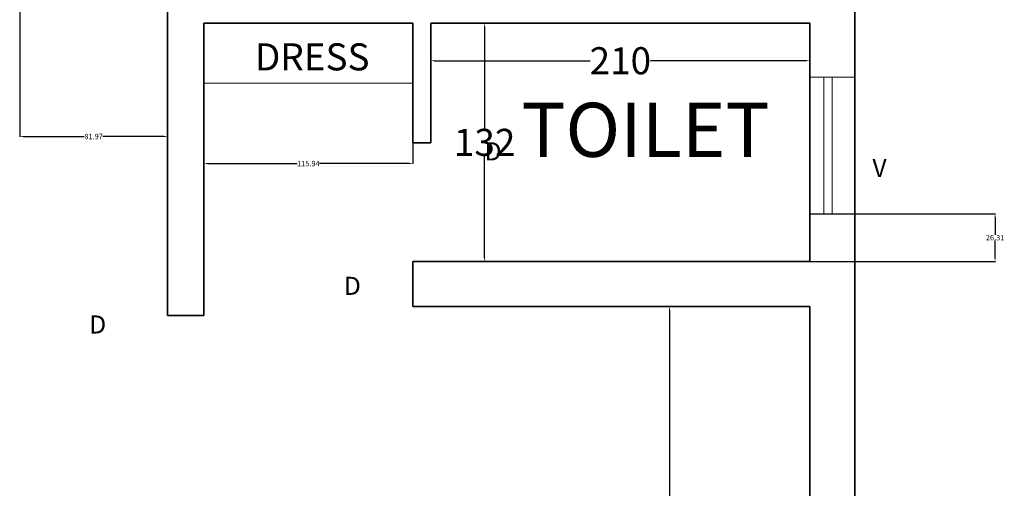
# Model space of a CAD drawing. Units: centimetres. Extents: x -121 to 3851, y -16 to 1180.
# Tile 8 of 16: x 958 to 1504, y 288 to 548. Entities that reach past the tile are written whole.
import ezdxf

# ---------------------------------------------------------------- set-up
doc = ezdxf.new("R2010")
doc.units = ezdxf.units.CM
doc.header["$MEASUREMENT"] = 0
for name, color, linetype, lineweight in [('A-ANNO-DIMS', 2, 'Continuous', 18), ('A-ANNO-IDEN', 3, 'Continuous', 13), ('A-AREA-IDEN', 3, 'Continuous', 18), ('A-FLOR-CASE', 9, 'Continuous', 18), ('A-GLAZ', 4, 'Continuous', 18), ('A-WALL', 7, 'Continuous', 35)]:
    doc.layers.add(name, color=color, linetype=linetype, lineweight=lineweight)
doc.styles.get("Standard").update_dxf_attribs({"font": 'arial.ttf'})
doc.dimstyles.get("Standard").update_dxf_attribs({"dimtxt": 3, "dimasz": 2, "dimexe": 0.18, "dimexo": 0.0625, "dimgap": 0.09, "dimtad": 0, "dimtih": 1, "dimtoh": 1, "dimdec": 0, "dimzin": 0, "dimdsep": 46, "dimtxsty": 'Standard', "dimcen": 0.09, "dimadec": 0, "dimazin": 0, "dimtfac": 1, "dimtdec": 0, "dimtofl": 0, "dimtmove": 0, "dimatfit": 3, "dimfxl": 1, "dimtolj": 1, "dimtzin": 0, "dimarcsym": 0})

# ---------------------------------------------------------------- blocks, each defined once
blk = doc.blocks.new('*D11')
at = {"layer": 'A-ANNO-DIMS', "color": 0, "lineweight": -2, "transparency": 16777216}
for p, q in [((1215.86, 546.01), (1215.98, 546.01)), ((1215.8, 544.01), (1215.8, 487.77)), ((1215.8, 416.01), (1215.8, 472.26)), ((1215.86, 414.01), (1215.98, 414.01))]:
    blk.add_line(p, q, dxfattribs=at)
at = {"layer": 'A-ANNO-DIMS', "color": 0, "transparency": 16777216}
for points in [[(1215.46, 544.01), (1216.13, 544.01), (1215.8, 546.01)], [(1215.46, 416.01), (1216.13, 416.01), (1215.8, 414.01)]]:
    blk.add_solid(points, dxfattribs=at)
at = {"layer": 'Defpoints', "color": 0, "transparency": 16777216}
for p in [(1215.8, 546.01), (1215.8, 414.01), (1215.8, 414.01)]:
    blk.add_point(p, dxfattribs=at)
at = {"layer": 'A-ANNO-DIMS', "color": 0, "transparency": 16777216, "insert": (1215.8, 480.01), "char_height": 3, "attachment_point": 5}
blk.add_mtext('\\A1;{\\H5x;132}', dxfattribs=at)
blk = doc.blocks.new('*D12')
at = {"layer": 'A-ANNO-DIMS', "color": 0, "lineweight": -2, "transparency": 16777216}
for p, q in [((1186.04, 520.45), (1186.04, 525.46)), ((1188.04, 525.28), (1274.28, 525.28)), ((1394.04, 525.28), (1307.8, 525.28)), ((1396.04, 520.45), (1396.04, 525.46))]:
    blk.add_line(p, q, dxfattribs=at)
at = {"layer": 'A-ANNO-DIMS', "color": 0, "transparency": 16777216}
for points in [[(1188.04, 525.62), (1188.04, 524.95), (1186.04, 525.28)], [(1394.04, 525.62), (1394.04, 524.95), (1396.04, 525.28)]]:
    blk.add_solid(points, dxfattribs=at)
at = {"layer": 'Defpoints', "color": 0, "transparency": 16777216}
for p in [(1396.04, 525.28), (1186.04, 520.39), (1396.04, 520.39)]:
    blk.add_point(p, dxfattribs=at)
at = {"layer": 'A-ANNO-DIMS', "color": 0, "transparency": 16777216, "insert": (1291.04, 525.28), "char_height": 3, "attachment_point": 5}
blk.add_mtext('\\A1;{\\H5x;210}', dxfattribs=at)
blk = doc.blocks.new('VENT-76CM')
for p, q in [((7.77, 75.86), (7.77, 0)), ((12.5, 75.86), (12.5, 0))]:
    blk.add_line(p, q)
blk.add_lwpolyline([(0, 75.86), (25, 75.86), (25, 0), (0, 0)], close=True)
blk = doc.blocks.new('*D52')
at = {"layer": 'A-ANNO-DIMS', "color": 0, "lineweight": -2, "transparency": 16777216}
for p, q in [((958.04, 560.95), (958.04, 483.08)), ((1040.01, 560.95), (1040.01, 483.08)), ((960.04, 483.26), (993.87, 483.26)), ((1038.01, 483.26), (1004.18, 483.26))]:
    blk.add_line(p, q, dxfattribs=at)
at = {"layer": 'A-ANNO-DIMS', "color": 0, "transparency": 16777216}
for points in [[(960.04, 483.6), (960.04, 482.93), (958.04, 483.26)], [(1038.01, 483.6), (1038.01, 482.93), (1040.01, 483.26)]]:
    blk.add_solid(points, dxfattribs=at)
at = {"layer": 'Defpoints', "color": 0, "transparency": 16777216}
for p in [(958.04, 561.01), (1040.01, 561.01), (958.04, 483.26)]:
    blk.add_point(p, dxfattribs=at)
at = {"layer": 'A-ANNO-DIMS', "color": 0, "transparency": 16777216, "insert": (999.02, 483.26), "char_height": 3, "attachment_point": 5}
blk.add_mtext('\\A1;81.97', dxfattribs=at)
blk = doc.blocks.new('*D54')
at = {"layer": 'A-ANNO-DIMS', "color": 0, "lineweight": -2, "transparency": 16777216}
for p, q in [((1396.1, 440.32), (1498.97, 440.32)), ((1498.79, 438.32), (1498.79, 428.79)), ((1498.79, 416.01), (1498.79, 425.55)), ((1396.1, 414.01), (1498.97, 414.01))]:
    blk.add_line(p, q, dxfattribs=at)
at = {"layer": 'A-ANNO-DIMS', "color": 0, "transparency": 16777216}
for points in [[(1498.45, 438.32), (1499.12, 438.32), (1498.79, 440.32)], [(1498.45, 416.01), (1499.12, 416.01), (1498.79, 414.01)]]:
    blk.add_solid(points, dxfattribs=at)
at = {"layer": 'Defpoints', "color": 0, "transparency": 16777216}
for p in [(1396.04, 440.32), (1498.79, 440.32), (1396.04, 414.01)]:
    blk.add_point(p, dxfattribs=at)
at = {"layer": 'A-ANNO-DIMS', "color": 0, "transparency": 16777216, "insert": (1498.79, 427.17), "char_height": 3, "attachment_point": 5}
blk.add_mtext('\\A1;26.31', dxfattribs=at)
blk = doc.blocks.new('*D61')
at = {"layer": 'A-ANNO-DIMS', "color": 0, "lineweight": -2, "transparency": 16777216}
for p, q in [((1395.98, 389.01), (1318.11, 389.01)), ((1318.29, 387.01), (1318.29, 240.64)), ((1318.29, 91.01), (1318.29, 237.39)), ((1395.98, 89.01), (1318.11, 89.01))]:
    blk.add_line(p, q, dxfattribs=at)
at = {"layer": 'A-ANNO-DIMS', "color": 0, "transparency": 16777216}
for points in [[(1317.95, 387.01), (1318.62, 387.01), (1318.29, 389.01)], [(1317.95, 91.01), (1318.62, 91.01), (1318.29, 89.01)]]:
    blk.add_solid(points, dxfattribs=at)
at = {"layer": 'Defpoints', "color": 0, "transparency": 16777216}
for p in [(1318.29, 389.01), (1396.04, 389.01), (1396.04, 89.01)]:
    blk.add_point(p, dxfattribs=at)
at = {"layer": 'A-ANNO-DIMS', "color": 0, "transparency": 16777216, "insert": (1318.29, 239.01), "char_height": 3, "attachment_point": 5}
blk.add_mtext('\\A1;300', dxfattribs=at)
blk = doc.blocks.new('*D62')
at = {"layer": 'A-ANNO-DIMS', "color": 0, "lineweight": -2, "transparency": 16777216}
for p, q in [((1060.1, 545.95), (1060.1, 468.08)), ((1176.04, 545.95), (1176.04, 468.08)), ((1062.1, 468.26), (1111.9, 468.26)), ((1174.04, 468.26), (1124.24, 468.26))]:
    blk.add_line(p, q, dxfattribs=at)
at = {"layer": 'A-ANNO-DIMS', "color": 0, "transparency": 16777216}
for points in [[(1062.1, 468.6), (1062.1, 467.93), (1060.1, 468.26)], [(1174.04, 468.6), (1174.04, 467.93), (1176.04, 468.26)]]:
    blk.add_solid(points, dxfattribs=at)
at = {"layer": 'Defpoints', "color": 0, "transparency": 16777216}
for p in [(1060.1, 546.01), (1176.04, 546.01), (1060.1, 468.26)]:
    blk.add_point(p, dxfattribs=at)
at = {"layer": 'A-ANNO-DIMS', "color": 0, "transparency": 16777216, "insert": (1118.07, 468.26), "char_height": 3, "attachment_point": 5}
blk.add_mtext('\\A1;115.94', dxfattribs=at)

msp = doc.modelspace()

# ---------------------------------------------------------------- linework, layer by layer
at = {"layer": 'A-FLOR-CASE'}
msp.add_line((1176.0382, 512.8348), (1060.101, 512.8348), dxfattribs=at)
at = {"layer": 'A-WALL'}
for p, q in [((1421.0382, 880.0141), (1421.0382, 64.0141)), ((1060.101, 546.0141), (1176.0382, 546.0141)), ((1176.0382, 546.0141), (1176.0382, 479.6555)), ((1186.0382, 546.0141), (1186.0382, 479.6555)), ((1186.0382, 546.0141), (1396.0382, 546.0141)), ((1396.0382, 546.0141), (1396.0382, 414.0141)), ((1186.0382, 479.6555), (1176.0382, 479.6555)), ((1176.0382, 414.0141), (1396.0382, 414.0141)), ((1176.0382, 414.0141), (1176.0382, 389.0141)), ((1176.0382, 389.0141), (1396.0382, 389.0141)), ((1396.0382, 389.0141), (1396.0382, 89.0141)), ((1040.0075, 384.0141), (1060.101, 384.0141))]:
    msp.add_line(p, q, dxfattribs=at)
for points in [[(1060.101, 561.0141), (1040.0075, 561.0141), (1040.0075, 384.0141)], [(1060.101, 384.0141), (1060.101, 546.0141)]]:
    msp.add_lwpolyline(points, dxfattribs=at)

# ---------------------------------------------------------------- block references
at = {"layer": 'A-GLAZ'}
msp.add_blockref('VENT-76CM', (1396.038, 440.323), dxfattribs=at)

# ---------------------------------------------------------------- texts
at = {"layer": 'A-ANNO-IDEN', "char_height": 10, "attachment_point": 1}
for s, insert in [('D', (1215.7968, 480.0141)), ('V', (1430.7879, 470.8096)), ('D', (1137.7846, 405.4487)), ('D', (996.6131, 384.0141))]:
    msp.add_mtext_dynamic_manual_height_columns(s, width=55.718495, gutter_width=1, heights=[0], dxfattribs=dict(at, insert=insert))
at = {"layer": 'A-AREA-IDEN', "attachment_point": 1}
for s, width, insert, char_height in [('DRESS', 14.894434, (1088.4647, 534.9179), 15), ('TOILET', 114.065148, (1236.0976, 501.9549), 30)]:
    msp.add_mtext_dynamic_manual_height_columns(s, width=width, gutter_width=1, heights=[0], dxfattribs=dict(at, insert=insert, char_height=char_height))

# ---------------------------------------------------------------- dimensions: what is measured, and where the dimension line sits
at = {"layer": 'A-ANNO-DIMS'}
for base, p1, p2, angle, override, picture, middle in [((958.0382, 483.2641), (1040.0075, 561.0141), (958.0382, 561.0141), 180, {"dimdec": 2, "dimlfac": 1, "dimrnd": 0, "dimzin": 0, "dimdsep": 46, "dimlunit": 2}, '*D52', (999.0228, 483.2641)), ((1060.101, 468.2641), (1176.0382, 546.0141), (1060.101, 546.0141), 180, {"dimdec": 2, "dimlfac": 1, "dimrnd": 0, "dimzin": 0, "dimdsep": 46, "dimlunit": 2}, '*D62', (1118.0696, 468.2641)), ((1498.7882, 440.3227), (1396.0382, 414.0141), (1396.0382, 440.3227), 90, {"dimdec": 2, "dimlfac": 1, "dimrnd": 0, "dimzin": 0, "dimdsep": 46, "dimlunit": 2}, '*D54', (1498.7882, 427.1684)), ((1318.2882, 389.0141), (1396.0382, 89.0141), (1396.0382, 389.0141), 90, {"dimdec": 0, "dimlfac": 1, "dimrnd": 0, "dimzin": 0, "dimdsep": 46, "dimlunit": 2}, '*D61', (1318.2882, 239.0141))]:
    dim = msp.add_linear_dim(base=base, p1=p1, p2=p2, angle=angle, dimstyle='Standard', override=override, dxfattribs=at)
    dim.commit()
    dim.dimension.update_dxf_attribs({"geometry": picture, "text_midpoint": middle})
dim = msp.add_linear_dim(base=(1215.7968, 414.0141), p1=(1215.7968, 546.0141), p2=(1215.7968, 414.0141), angle=90, text='{\\H5x;<>}', dimstyle='Standard', override={"dimclrd": 0, "dimclre": 0, "dimclrt": 0}, dxfattribs=at)
dim.commit()
dim.dimension.update_dxf_attribs({"geometry": '*D11', "text_midpoint": (1215.7968, 480.0141)})
dim = msp.add_linear_dim(base=(1396.0382, 525.2845), p1=(1186.0382, 520.3903), p2=(1396.0382, 520.3903), text='{\\H5x;<>}', dimstyle='Standard', override={"dimclrd": 0, "dimclre": 0, "dimclrt": 0}, dxfattribs=at)
dim.commit()
dim.dimension.update_dxf_attribs({"geometry": '*D12', "text_midpoint": (1291.0382, 525.2845)})

doc.saveas('drawing.dxf')
